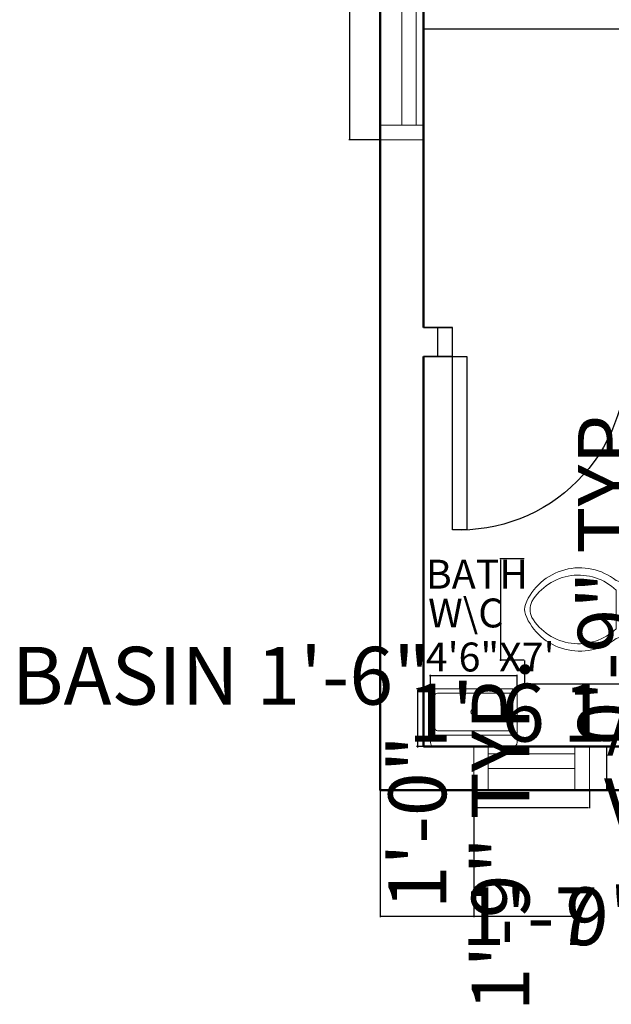
# Model space of a CAD drawing. Units: inches. Extents: x -52 to 472, y -40 to 644.
# Tile 1 of 6: x -52 to 71, y -40 to 164. Entities that reach past the tile are written whole.
import ezdxf

# ---------------------------------------------------------------- set-up
doc = ezdxf.new("R2010")
doc.units = ezdxf.units.IN
doc.header["$MEASUREMENT"] = 0
for name, color, linetype, lineweight in [('A-ANNO-DIMS', 7, 'Continuous', 13), ('A-ANNO-TEXT', 7, 'Continuous', 18), ('DOORS', 2, 'Continuous', 25), ('INNER WALL', 1, 'Continuous', 35), ('OUTER WALL', 1, 'Continuous', 50), ('S-PLUM', 151, 'Continuous', 18), ('VENTILATOR', 4, 'Continuous', 20), ('WINDOWS', 4, 'Continuous', 20)]:
    doc.layers.add(name, color=color, linetype=linetype, lineweight=lineweight)
doc.styles.get("Standard").update_dxf_attribs({"font": 'arial.ttf'})
doc.dimstyles.get("Standard").update_dxf_attribs({"dimtxt": 12, "dimasz": 0.18, "dimexe": 0.18, "dimexo": 0.0625, "dimgap": 0.09, "dimtad": 0, "dimdec": 1, "dimzin": 0, "dimdsep": 46, "dimlunit": 3, "dimtxsty": 'Standard', "dimcen": 0.09, "dimadec": 0, "dimazin": 0, "dimtfac": 1, "dimtdec": 1, "dimtofl": 0, "dimtmove": 0, "dimatfit": 3, "dimfxl": 1, "dimtolj": 1, "dimtzin": 0, "dimarcsym": 0})

# ---------------------------------------------------------------- blocks, each defined once
blk = doc.blocks.new('Toilet - top')
for p, q in [((9.5, -6), (9.5, -2)), ((-8, -8.5), (-8, -8)), ((-7, -8), (-7, -9.5)), ((-4, -8), (-6, -14)), ((4, -8), (6, -14)), ((-10, -8.5), (-8, -8.5)), ((-10, -9.5), (-10, -8.5)), ((-7, -9.5), (-10, -9.5)), ((4, -14), (-4, -14))]:
    blk.add_line(p, q)
blk.add_lwpolyline([(10.5, -8), (10.5, 0), (-10.5, 0), (-10.5, -8)], close=True)
for points in [[(-9.5, -2), (-9.5, -6)], [(8.5, -1), (-8.5, -1)], [(-8.5, -7), (8.5, -7)]]:
    blk.add_lwpolyline(points)
for centre, radius, start, end in [((-8.62, -1.88), 0.884, 81.8699, 188.1301), ((8.62, -1.88), 0.884, 351.8699, 98.1301), ((-8.62, -6.12), 0.884, 171.8699, 278.1301), ((8.62, -6.12), 0.884, 261.8699, 8.1301), ((3.52, -21.58), 12.17, 141.4691, 247.9714), ((4.2, -21.82), 11.33, 136.3677, 238.9468), ((-3.52, -21.58), 12.17, 292.0284, 38.5307), ((-4.2, -21.82), 11.33, 301.053, 43.6321), ((0, -27.88), 4, 245.7318, 294.2682), ((0, -29), 4, 254.8605, 285.1395)]:
    blk.add_arc(centre, radius, start, end)
blk = doc.blocks.new('*D17')
at = {"layer": 'A-ANNO-DIMS', "color": 0, "lineweight": -2, "transparency": 16777216}
for p, q in [((32.13, 162.39), (32.13, 162.51)), ((32.31, 162.33), (89.84, 162.33)), ((210.95, 162.33), (153.42, 162.33)), ((211.13, 162.39), (211.13, 162.51))]:
    blk.add_line(p, q, dxfattribs=at)
at = {"layer": 'A-ANNO-DIMS', "color": 0, "transparency": 16777216}
for points in [[(32.31, 162.36), (32.31, 162.3), (32.13, 162.33)], [(210.95, 162.36), (210.95, 162.3), (211.13, 162.33)]]:
    blk.add_solid(points, dxfattribs=at)
at = {"layer": 'Defpoints', "color": 0, "transparency": 16777216}
for p in [(32.13, 162.33), (32.13, 162.33), (211.13, 162.33)]:
    blk.add_point(p, dxfattribs=at)
at = {"layer": 'A-ANNO-DIMS', "color": 0, "transparency": 16777216, "insert": (121.63, 162.33), "char_height": 12, "attachment_point": 5}
blk.add_mtext('\\A1;14\'-11.0"', dxfattribs=at)
blk = doc.blocks.new('Sink-single - 30 in top')
blk.add_line((-15, -3.999996), (15, -3.999996))
for points in [[(-13.5, 0), (13.5, 0)], [(-15, -18.499996), (-15, -1.5)], [(15, -1.5), (15, -18.499996)], [(-13.5, -17.499996), (-13.5, -6.499996)], [(-12.5, -5.499996), (12.5, -5.499996)], [(13.5, -6.499996), (13.5, -17.499996)], [(13.5, -19.999996), (-13.5, -19.999996)], [(12.5, -18.499996), (-12.5, -18.499996)]]:
    blk.add_lwpolyline(points)
for radius in [1, 0.5]:
    blk.add_circle((0, -11.999996), radius)
for centre, radius, start, end in [((-13.5, -1.5), 1.5, 90, 180), ((13.5, -1.5), 1.5, 0, 90), ((-12.5, -6.499996), 1, 90, 180), ((12.5, -6.499996), 1, 0, 90), ((-13.5, -18.499996), 1.5, 180, 270), ((-12.5, -17.499996), 1, 180, 270), ((12.5, -17.499996), 1, 270, 0), ((13.5, -18.499996), 1.5, 270, 0)]:
    blk.add_arc(centre, radius, start, end)
blk = doc.blocks.new('WIN-36IN')
for p, q in [((9, 42), (0, 42)), ((9, 39), (0, 39)), ((4.5, 3), (4.5, 39)), ((7.5, 3), (7.5, 39)), ((0, 3), (9, 3)), ((0, 0), (9, 0))]:
    blk.add_line(p, q)
blk = doc.blocks.new('VENT-18IN')
for p, q in [((0, 9), (0, 0)), ((3, 9), (3, 0)), ((21, 0), (21, 9)), ((24, 0), (24, 9)), ((21, 7.5), (3, 7.5)), ((21, 4.5), (3, 4.5))]:
    blk.add_line(p, q)
blk = doc.blocks.new('DOOR-36IN-SINGLE')
for p, q in [((0, 6), (0, 0)), ((3, 6), (3, 0)), ((39, 6), (39, 0)), ((42, 6), (42, 0))]:
    blk.add_line(p, q)
blk.add_lwpolyline([(3, 6), (6, 6), (6, 42), (3, 42)], close=True)
blk.add_arc((4.5, 7.5), 34.53, 357.5104, 92.4896)
blk = doc.blocks.new('*D26')
at = {"layer": 'A-ANNO-DIMS', "color": 0, "lineweight": -2, "transparency": 16777216}
for p, q in [((23.07, 181.31), (16.65, 181.31)), ((16.83, 181.31), (16.83, 181.49)), ((16.83, 139.49), (16.83, 181.13)), ((23.07, 139.31), (16.65, 139.31))]:
    blk.add_line(p, q, dxfattribs=at)
at = {"layer": 'A-ANNO-DIMS', "color": 0, "transparency": 16777216}
for points in [[(16.8, 181.13), (16.86, 181.13), (16.83, 181.31)], [(16.8, 139.49), (16.86, 139.49), (16.83, 139.31)]]:
    blk.add_solid(points, dxfattribs=at)
at = {"layer": 'Defpoints', "color": 0, "transparency": 16777216}
for p in [(16.83, 181.31), (23.13, 181.31), (23.13, 139.31)]:
    blk.add_point(p, dxfattribs=at)
at = {"layer": 'A-ANNO-DIMS', "color": 0, "transparency": 16777216, "insert": (16.83, 257.5), "char_height": 12, "attachment_point": 5, "rotation": 90}
blk.add_mtext('\\A1;WINDOW 3\'-6" TYP.', dxfattribs=at)
blk = doc.blocks.new('*D34')
at = {"layer": 'A-ANNO-DIMS', "color": 0, "lineweight": -2, "transparency": 16777216}
for p, q in [((33.55, 28.05), (33.37, 28.05)), ((33.55, 25.41), (33.55, 28.23)), ((51.4, 28.05), (33.73, 28.05)), ((51.58, 25.41), (51.58, 28.23))]:
    blk.add_line(p, q, dxfattribs=at)
at = {"layer": 'A-ANNO-DIMS', "color": 0, "transparency": 16777216}
for points in [[(33.73, 28.08), (33.73, 28.02), (33.55, 28.05)], [(51.4, 28.08), (51.4, 28.02), (51.58, 28.05)]]:
    blk.add_solid(points, dxfattribs=at)
at = {"layer": 'Defpoints', "color": 0, "transparency": 16777216}
for p in [(33.55, 28.05), (33.55, 25.34), (51.58, 25.34)]:
    blk.add_point(p, dxfattribs=at)
at = {"layer": 'A-ANNO-DIMS', "color": 0, "transparency": 16777216, "insert": (-9.88, 28.05), "char_height": 12, "attachment_point": 5}
blk.add_mtext('\\A1;BASIN 1\'-6"', dxfattribs=at)
blk = doc.blocks.new('*D35')
at = {"layer": 'A-ANNO-DIMS', "color": 0, "lineweight": -2, "transparency": 16777216}
for p, q in [((33.49, 25.34), (30.67, 25.34)), ((30.85, 25.16), (30.85, 13.51)), ((33.49, 13.33), (30.67, 13.33)), ((30.85, 13.33), (30.85, 13.15))]:
    blk.add_line(p, q, dxfattribs=at)
at = {"layer": 'A-ANNO-DIMS', "color": 0, "transparency": 16777216}
for points in [[(30.82, 25.16), (30.88, 25.16), (30.85, 25.34)], [(30.82, 13.51), (30.88, 13.51), (30.85, 13.33)]]:
    blk.add_solid(points, dxfattribs=at)
at = {"layer": 'Defpoints', "color": 0, "transparency": 16777216}
for p in [(33.55, 25.34), (30.85, 13.33), (33.55, 13.33)]:
    blk.add_point(p, dxfattribs=at)
at = {"layer": 'A-ANNO-DIMS', "color": 0, "transparency": 16777216, "insert": (30.85, -2.33), "char_height": 12, "attachment_point": 5, "rotation": 90}
blk.add_mtext('\\A1;1\'-0"', dxfattribs=at)
blk = doc.blocks.new('*D46')
at = {"layer": 'A-ANNO-DIMS', "color": 0, "lineweight": -2, "transparency": 16777216}
for p, q in [((53.09, 31.25), (53.09, 26.17)), ((86.13, 31.25), (86.13, 26.17)), ((53.27, 26.35), (85.95, 26.35)), ((86.13, 26.35), (86.31, 26.35))]:
    blk.add_line(p, q, dxfattribs=at)
at = {"layer": 'A-ANNO-DIMS', "color": 0, "transparency": 16777216}
for points in [[(53.27, 26.38), (53.27, 26.32), (53.09, 26.35)], [(85.95, 26.38), (85.95, 26.32), (86.13, 26.35)]]:
    blk.add_solid(points, dxfattribs=at)
at = {"layer": 'Defpoints', "color": 0, "transparency": 16777216}
for p in [(53.09, 31.31), (86.13, 31.31), (86.13, 26.35)]:
    blk.add_point(p, dxfattribs=at)
at = {"layer": 'A-ANNO-DIMS', "color": 0, "transparency": 16777216, "insert": (139.51, 26.35), "char_height": 12, "attachment_point": 5}
blk.add_mtext('\\A1;WC 2\'-9" TYP.', dxfattribs=at)
blk = doc.blocks.new('*D47')
at = {"layer": 'A-ANNO-DIMS', "color": 0, "lineweight": -2, "transparency": 16777216}
for p, q in [((53.02, 52.31), (47.95, 52.31)), ((48.13, 52.13), (48.13, 31.49)), ((53.02, 31.31), (47.95, 31.31)), ((48.13, 31.31), (48.13, 31.13))]:
    blk.add_line(p, q, dxfattribs=at)
at = {"layer": 'A-ANNO-DIMS', "color": 0, "transparency": 16777216}
for points in [[(48.1, 52.13), (48.16, 52.13), (48.13, 52.31)], [(48.1, 31.49), (48.16, 31.49), (48.13, 31.31)]]:
    blk.add_solid(points, dxfattribs=at)
at = {"layer": 'Defpoints', "color": 0, "transparency": 16777216}
for p in [(53.09, 52.31), (48.13, 31.31), (53.09, 31.31)]:
    blk.add_point(p, dxfattribs=at)
at = {"layer": 'A-ANNO-DIMS', "color": 0, "transparency": 16777216, "insert": (48.13, -4.97), "char_height": 12, "attachment_point": 5, "rotation": 90}
blk.add_mtext('\\A1;1\'-9" TYP.', dxfattribs=at)
blk = doc.blocks.new('*D48')
at = {"layer": 'A-ANNO-DIMS', "color": 0, "lineweight": -2, "transparency": 16777216}
for p, q in [((42.57, 4.27), (42.57, 0.55)), ((66.57, 4.27), (66.57, 0.55)), ((42.75, 0.73), (66.39, 0.73)), ((66.57, 0.73), (66.75, 0.73))]:
    blk.add_line(p, q, dxfattribs=at)
at = {"layer": 'A-ANNO-DIMS', "color": 0, "transparency": 16777216}
for points in [[(42.75, 0.76), (42.75, 0.7), (42.57, 0.73)], [(66.39, 0.76), (66.39, 0.7), (66.57, 0.73)]]:
    blk.add_solid(points, dxfattribs=at)
at = {"layer": 'Defpoints', "color": 0, "transparency": 16777216}
for p in [(42.57, 4.33), (66.57, 4.33), (66.57, 0.73)]:
    blk.add_point(p, dxfattribs=at)
at = {"layer": 'A-ANNO-DIMS', "color": 0, "transparency": 16777216, "insert": (128.4, 0.73), "char_height": 12, "attachment_point": 5}
blk.add_mtext('\\A1;VENT 2\'-0" TYP.', dxfattribs=at)
blk = doc.blocks.new('*D49')
at = {"layer": 'A-ANNO-DIMS', "color": 0, "lineweight": -2, "transparency": 16777216}
for p, q in [((66.63, 13.33), (70.35, 13.33)), ((70.17, 13.33), (70.17, 13.51)), ((70.17, 4.51), (70.17, 13.15)), ((66.63, 4.33), (70.35, 4.33))]:
    blk.add_line(p, q, dxfattribs=at)
at = {"layer": 'A-ANNO-DIMS', "color": 0, "transparency": 16777216}
for points in [[(70.14, 13.15), (70.2, 13.15), (70.17, 13.33)], [(70.14, 4.51), (70.2, 4.51), (70.17, 4.33)]]:
    blk.add_solid(points, dxfattribs=at)
at = {"layer": 'Defpoints', "color": 0, "transparency": 16777216}
for p in [(66.57, 13.33), (70.17, 13.33), (66.57, 4.33)]:
    blk.add_point(p, dxfattribs=at)
at = {"layer": 'A-ANNO-DIMS', "color": 0, "transparency": 16777216, "insert": (70.17, 50.17), "char_height": 12, "attachment_point": 5, "rotation": 90}
blk.add_mtext('\\A1;0\'-9" TYP.', dxfattribs=at)
blk = doc.blocks.new('*D58')
at = {"layer": 'A-ANNO-DIMS', "color": 0, "lineweight": -2, "transparency": 16777216}
for p, q in [((90.73, 69.61), (84.19, 69.61)), ((84.37, 69.61), (84.37, 69.79)), ((84.37, 26.98), (84.37, 69.43)), ((90.73, 26.8), (84.19, 26.8))]:
    blk.add_line(p, q, dxfattribs=at)
at = {"layer": 'A-ANNO-DIMS', "color": 0, "transparency": 16777216}
for points in [[(84.34, 69.43), (84.4, 69.43), (84.37, 69.61)], [(84.34, 26.98), (84.4, 26.98), (84.37, 26.8)]]:
    blk.add_solid(points, dxfattribs=at)
at = {"layer": 'Defpoints', "color": 0, "transparency": 16777216}
for p in [(84.37, 69.61), (90.79, 69.61), (90.79, 26.8)]:
    blk.add_point(p, dxfattribs=at)
at = {"layer": 'A-ANNO-DIMS', "color": 0, "transparency": 16777216, "insert": (84.37, 110.95), "char_height": 12, "attachment_point": 5, "rotation": 90}
blk.add_mtext('\\A1;SOFA 3\'-7"', dxfattribs=at)
blk = doc.blocks.new('*D59')
at = {"layer": 'A-ANNO-DIMS', "color": 0, "lineweight": -2, "transparency": 16777216}
for p, q in [((90.79, 26.74), (90.79, 20.2)), ((109.47, 26.74), (109.47, 20.2)), ((90.79, 20.38), (90.61, 20.38)), ((109.29, 20.38), (90.97, 20.38))]:
    blk.add_line(p, q, dxfattribs=at)
at = {"layer": 'A-ANNO-DIMS', "color": 0, "transparency": 16777216}
for points in [[(90.97, 20.41), (90.97, 20.35), (90.79, 20.38)], [(109.29, 20.41), (109.29, 20.35), (109.47, 20.38)]]:
    blk.add_solid(points, dxfattribs=at)
at = {"layer": 'Defpoints', "color": 0, "transparency": 16777216}
for p in [(90.79, 26.8), (109.47, 26.8), (90.79, 20.38)]:
    blk.add_point(p, dxfattribs=at)
at = {"layer": 'A-ANNO-DIMS', "color": 0, "transparency": 16777216, "insert": (61.15, 20.38), "char_height": 12, "attachment_point": 5}
blk.add_mtext('\\A1;1\'-6 1/2"', dxfattribs=at)
blk = doc.blocks.new('*D75')
at = {"layer": 'A-ANNO-DIMS', "color": 0, "lineweight": -2, "transparency": 16777216}
for p, q in [((23.13, 4.27), (23.13, -22.05)), ((136.13, 4.27), (136.13, -22.05)), ((23.31, -21.87), (63.59, -21.87)), ((135.95, -21.87), (95.67, -21.87))]:
    blk.add_line(p, q, dxfattribs=at)
at = {"layer": 'A-ANNO-DIMS', "color": 0, "transparency": 16777216}
for points in [[(23.31, -21.84), (23.31, -21.9), (23.13, -21.87)], [(135.95, -21.84), (135.95, -21.9), (136.13, -21.87)]]:
    blk.add_solid(points, dxfattribs=at)
at = {"layer": 'Defpoints', "color": 0, "transparency": 16777216}
for p in [(23.13, 4.33), (136.13, 4.33), (136.13, -21.87)]:
    blk.add_point(p, dxfattribs=at)
at = {"layer": 'A-ANNO-DIMS', "color": 0, "transparency": 16777216, "insert": (79.63, -21.87), "char_height": 12, "attachment_point": 5}
blk.add_mtext('\\A1;9\'-5"', dxfattribs=at)
blk = doc.blocks.new('*D76')
at = {"layer": 'A-ANNO-DIMS', "color": 0, "lineweight": -2, "transparency": 16777216}
for p, q in [((23.13, 4.27), (23.13, -22.05)), ((42.57, 4.27), (42.57, -22.05)), ((23.31, -21.87), (42.39, -21.87)), ((42.57, -21.87), (42.75, -21.87))]:
    blk.add_line(p, q, dxfattribs=at)
at = {"layer": 'A-ANNO-DIMS', "color": 0, "transparency": 16777216}
for points in [[(23.31, -21.84), (23.31, -21.9), (23.13, -21.87)], [(42.39, -21.84), (42.39, -21.9), (42.57, -21.87)]]:
    blk.add_solid(points, dxfattribs=at)
at = {"layer": 'Defpoints', "color": 0, "transparency": 16777216}
for p in [(23.13, 4.33), (42.57, 4.33), (42.57, -21.87)]:
    blk.add_point(p, dxfattribs=at)
at = {"layer": 'A-ANNO-DIMS', "color": 0, "transparency": 16777216, "insert": (72.2, -21.87), "char_height": 12, "attachment_point": 5}
blk.add_mtext('\\A1;1\'-7 1/2"', dxfattribs=at)

msp = doc.modelspace()

# ---------------------------------------------------------------- linework, layer by layer
at = {"layer": 'INNER WALL'}
for p, q in [((38.13, 100.33), (32.13, 100.33)), ((38.13, 94.33), (32.13, 94.33))]:
    msp.add_line(p, q, dxfattribs=at)
at = {"layer": 'OUTER WALL'}
for p, q in [((32.13, 210.33), (32.13, 100.33)), ((32.13, 94.33), (32.13, 13.33)), ((32.13, 13.33), (86.13, 13.33))]:
    msp.add_line(p, q, dxfattribs=at)
msp.add_lwpolyline([(208.13, 4.33), (353.13, 4.33), (353.13, 482.33), (23.13, 482.33), (23.13, 4.33), (136.13, 4.33)], dxfattribs=at)

# ---------------------------------------------------------------- block references
at = {"layer": 'DOORS', "extrusion": (0, 0, -1), "zscale": -1, "rotation": 180}
msp.add_blockref('DOOR-36IN-SINGLE', (-35.13, 100.33), dxfattribs=at)
at = {"layer": 'S-PLUM', "rotation": 270}
msp.add_blockref('Toilet - top', (86.13, 41.81), dxfattribs=at)
at = {"layer": 'S-PLUM', "xscale": 0.6007315394121483, "yscale": 0.6007315394121483, "zscale": 0.6007315394121483, "rotation": 180}
msp.add_blockref('Sink-single - 30 in top', (42.57, 13.33), dxfattribs=at)
at = {"layer": 'VENTILATOR'}
msp.add_blockref('VENT-18IN', (42.57, 4.33), dxfattribs=at)
at = {"layer": 'WINDOWS'}
msp.add_blockref('WIN-36IN', (23.13, 139.31), dxfattribs=at)

# ---------------------------------------------------------------- texts
at = {"layer": 'A-ANNO-TEXT'}
for s, p in [('BATH', (32.62, 46.13)), ('W\\C', (33.09, 38.08)), ('4\'6"X7\'', (32.59, 28.94))]:
    msp.add_text(s, height=6, dxfattribs=at).set_placement(p)

# ---------------------------------------------------------------- dimensions: what is measured, and where the dimension line sits
at = {"layer": 'A-ANNO-DIMS'}
for base, p1, p2, angle, text, picture, middle in [((16.83, 181.31), (23.13, 139.31), (23.13, 181.31), 90, 'WINDOW <> TYP.', '*D26', (16.83, 257.5)), ((84.37, 69.61), (90.79, 26.8), (90.79, 69.61), 90, 'SOFA <>', '*D58', (84.37, 110.95)), ((70.17, 13.33), (66.57, 4.33), (66.57, 13.33), 90, '<> TYP.', '*D49', (70.17, 50.17)), ((48.13, 31.31), (53.09, 52.31), (53.09, 31.31), 270, '<> TYP.', '*D47', (48.13, -4.97)), ((33.55, 28.05), (51.58, 25.34), (33.55, 25.34), 180, 'BASIN <>', '*D34', (-9.88, 28.05))]:
    dim = msp.add_linear_dim(base=base, p1=p1, p2=p2, angle=angle, text=text, dimstyle='Standard', override={"dimdec": 1, "dimlfac": 1, "dimrnd": 0, "dimzin": 1, "dimdsep": 46, "dimlunit": 4, "dimfrac": 2}, dxfattribs=at)
    dim.commit()
    dim.dimension.update_dxf_attribs({"geometry": picture, "text_midpoint": middle})
for base, p1, p2, override, picture, middle in [((32.13, 162.33), (211.13, 162.33), (32.13, 162.33), {"dimclrd": 0, "dimclre": 0, "dimclrt": 0}, '*D17', (121.63, 162.33)), ((136.13, -21.87), (23.13, 4.33), (136.13, 4.33), {"dimdec": 1, "dimlfac": 1, "dimrnd": 0, "dimzin": 1, "dimdsep": 46, "dimlunit": 4, "dimfrac": 2}, '*D75', (79.63, -21.87)), ((42.57, -21.87), (23.13, 4.33), (42.57, 4.33), {"dimdec": 1, "dimlfac": 1, "dimrnd": 0, "dimzin": 1, "dimdsep": 46, "dimlunit": 4, "dimfrac": 2}, '*D76', (72.2, -21.87))]:
    dim = msp.add_linear_dim(base=base, p1=p1, p2=p2, dimstyle='Standard', override=override, dxfattribs=at)
    dim.commit()
    dim.dimension.update_dxf_attribs({"geometry": picture, "text_midpoint": middle})
for base, p1, p2, text, picture, middle in [((86.13, 26.35), (53.09, 31.31), (86.13, 31.31), 'WC <> TYP.', '*D46', (139.51, 26.35)), ((66.57, 0.73), (42.57, 4.33), (66.57, 4.33), 'VENT <> TYP.', '*D48', (128.4, 0.73))]:
    dim = msp.add_linear_dim(base=base, p1=p1, p2=p2, text=text, dimstyle='Standard', override={"dimdec": 1, "dimlfac": 1, "dimrnd": 0, "dimzin": 1, "dimdsep": 46, "dimlunit": 4, "dimfrac": 2}, dxfattribs=at)
    dim.commit()
    dim.dimension.update_dxf_attribs({"geometry": picture, "text_midpoint": middle})
for base, p1, p2, angle, picture, middle in [((90.79, 20.38), (109.47, 26.8), (90.79, 26.8), 180, '*D59', (61.15, 20.38)), ((30.85, 13.33), (33.55, 25.34), (33.55, 13.33), 270, '*D35', (30.85, -2.33))]:
    dim = msp.add_linear_dim(base=base, p1=p1, p2=p2, angle=angle, dimstyle='Standard', override={"dimdec": 1, "dimlfac": 1, "dimrnd": 0, "dimzin": 1, "dimdsep": 46, "dimlunit": 4, "dimfrac": 2}, dxfattribs=at)
    dim.commit()
    dim.dimension.update_dxf_attribs({"geometry": picture, "text_midpoint": middle})

doc.saveas('drawing.dxf')
